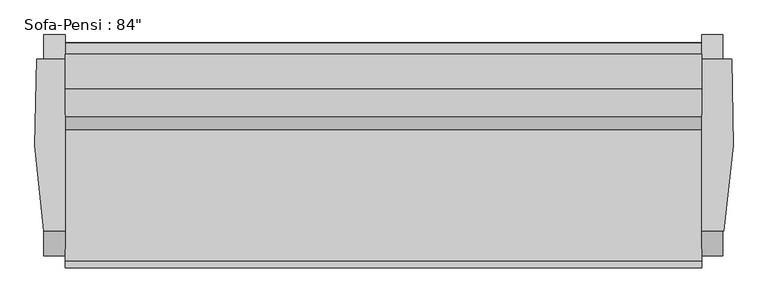
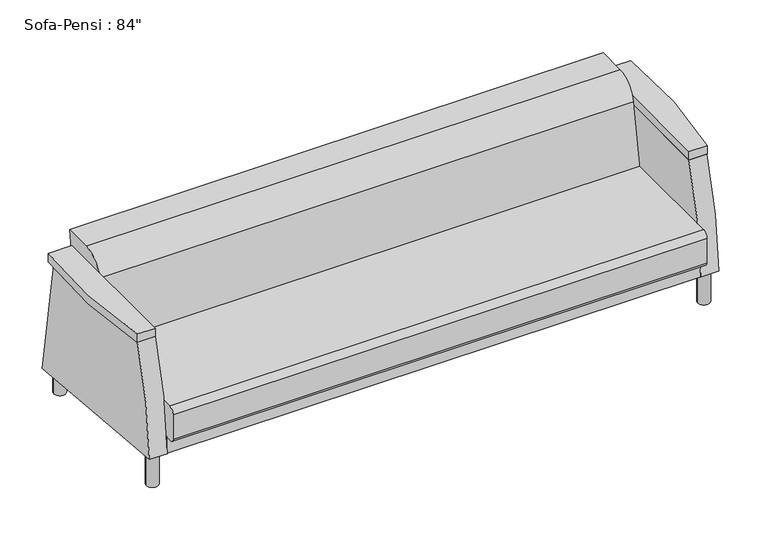
"""IFC4 building model written with IfcOpenShell, lengths in millimetres: furniture geometry."""

from ifc_helpers import new_model, si_unit, point, frame, frame_2d, origin, origin_with_axes, place, context, project, spatial, polyline, circle_curve, trimmed, segment, composite_curve, outline, extrude, source, transform, mapped, element, save


def furniture_1a2ca15e(model_context):
    return source(origin(), model_context, "Body", "SweptSolid", [
        extrude(outline(composite_curve([segment(trimmed(circle_curve(frame_2d((-902.49375, -53.0901639)), 25.4), [point((-927.89375, -53.0901639))], [point((-877.09375, -53.0901639))], False, "CARTESIAN"), True, "CONTINUOUS"), segment(trimmed(circle_curve(frame_2d((-902.49375, -53.0901639)), 25.4), [point((-877.09375, -53.0901639))], [point((-927.89375, -53.0901639))], False, "CARTESIAN"), True, "CONTINUOUS")], self_intersect=False)), origin_with_axes(), (0.0, 0.0, 1.0), 148.43125),
        extrude(outline(composite_curve([segment(trimmed(circle_curve(frame_2d((-902.49375, 632.7098361)), 25.4), [point((-927.89375, 632.7098361))], [point((-877.09375, 632.7098361))], False, "CARTESIAN"), True, "CONTINUOUS"), segment(trimmed(circle_curve(frame_2d((-902.49375, 632.7098361)), 25.4), [point((-877.09375, 632.7098361))], [point((-927.89375, 632.7098361))], False, "CARTESIAN"), True, "CONTINUOUS")], self_intersect=False)), origin_with_axes(), (0.0, 0.0, 1.0), 148.43125),
        extrude(outline(composite_curve([segment(trimmed(circle_curve(frame_2d((1459.70625, 632.7098361)), 25.4), [point((1434.30625, 632.7098361))], [point((1485.10625, 632.7098361))], False, "CARTESIAN"), True, "CONTINUOUS"), segment(trimmed(circle_curve(frame_2d((1459.70625, 632.7098361)), 25.4), [point((1485.10625, 632.7098361))], [point((1434.30625, 632.7098361))], False, "CARTESIAN"), True, "CONTINUOUS")], self_intersect=False)), origin_with_axes(), (0.0, 0.0, 1.0), 148.43125),
        extrude(outline(composite_curve([segment(trimmed(circle_curve(frame_2d((1459.70625, -53.0901639)), 25.4), [point((1434.30625, -53.0901639))], [point((1485.10625, -53.0901639))], False, "CARTESIAN"), True, "CONTINUOUS"), segment(trimmed(circle_curve(frame_2d((1459.70625, -53.0901639)), 25.4), [point((1485.10625, -53.0901639))], [point((1434.30625, -53.0901639))], False, "CARTESIAN"), True, "CONTINUOUS")], self_intersect=False)), origin_with_axes(), (0.0, 0.0, 1.0), 148.43125),
        extrude(outline(polyline([(1421.60625, 668.3047863), (1421.60625, -93.6952137), (-864.39375, -93.6952137), (-864.39375, 668.3047863), (1421.60625, 668.3047863)])), frame((0.0, 0.0, 148.0509954), z_axis=(0.0, 0.0, 1.0), x_axis=(1.0, 0.0, 0.0)), (0.0, 0.0, 1.0), 76.2),
        extrude(outline(composite_curve([segment(polyline([(-9.3943348, 626.0203985), (608.6917937, 626.0203985), (696.2098361, 79.844579), (-97.7900405, 149.3105671)]), True, "CONTINUOUS"), segment(trimmed(circle_curve(frame_2d((1499.9783711, 99.5888442)), 1598.5418814), [point((-97.7900405, 149.3105671))], [point((-9.3943348, 626.0203985))], False, "CARTESIAN"), True, "CONTINUOUS")], self_intersect=False)), frame((-940.59375, 0.0, 0.0), z_axis=(1.0, 0.0, 0.0), x_axis=(0.0, 1.0, 0.0)), (0.0, 0.0, 1.0), 76.2),
        extrude(outline(composite_curve([segment(polyline([(696.2098361, 79.844579), (-97.7900405, 149.3105671)]), True, "CONTINUOUS"), segment(trimmed(circle_curve(frame_2d((1499.9783711, 99.5888442)), 1598.5418814), [point((-97.7900405, 149.3105671))], [point((-9.3943348, 626.0203985))], False, "CARTESIAN"), True, "CONTINUOUS"), segment(polyline([(-9.3943348, 626.0203985), (608.6917937, 626.0203985), (696.2098361, 79.844579)]), True, "CONTINUOUS")], self_intersect=False)), frame((1421.60625, 0.0, 0.0), z_axis=(1.0, 0.0, 0.0), x_axis=(0.0, 1.0, 0.0)), (0.0, 0.0, 1.0), 76.2),
        extrude(outline(composite_curve([segment(trimmed(circle_curve(frame_2d((-116.5901639, 351.2509954)), 25.4), [point((-141.9901639, 351.2509954))], [point((-116.5901639, 376.6509954))], False, "CARTESIAN"), True, "CONTINUOUS"), segment(polyline([(-116.5901639, 376.6509954), (355.3895541, 376.6509954), (402.1988177, 642.1195211)]), True, "CONTINUOUS"), segment(trimmed(circle_curve(frame_2d((502.2552854, 624.4768662)), 101.6), [point((402.1988177, 642.1195211))], [point((502.2552854, 726.0768662))], False, "CARTESIAN"), True, "CONTINUOUS"), segment(polyline([(502.2552854, 726.0768662), (626.3344485, 726.0768662), (609.5377828, 620.1719187), (667.6541767, 224.2509954), (-126.1151639, 224.2509954)]), True, "CONTINUOUS"), segment(trimmed(circle_curve(frame_2d((-126.1151639, 240.1259954)), 15.875), [point((-126.1151639, 224.2509954))], [point((-141.9901639, 240.1259954))], False, "CARTESIAN"), True, "CONTINUOUS"), segment(polyline([(-141.9901639, 240.1259954), (-141.9901639, 351.2509954)]), True, "CONTINUOUS")], self_intersect=False)), frame((-864.39375, 0.0, 0.0), z_axis=(1.0, 0.0, 0.0), x_axis=(0.0, 1.0, 0.0)), (0.0, 0.0, 1.0), 2286.0),
        extrude(outline(composite_curve([segment(polyline([(-864.39375, -9.3943348), (-940.59375, -9.3943348)]), True, "CONTINUOUS"), segment(trimmed(circle_curve(frame_2d((1531.9527561, 401.7789315)), 2506.5014821), [point((-940.59375, -9.3943348))], [point((-965.99375, 608.6917935))], False, "CARTESIAN"), True, "CONTINUOUS"), segment(polyline([(-965.99375, 608.6917935), (-864.39375, 608.6917935), (-864.39375, -9.3943348)]), True, "CONTINUOUS")], self_intersect=False)), frame((0.0, 0.0, 626.0203985), z_axis=(0.0, 0.0, 1.0), x_axis=(1.0, 0.0, 0.0)), (0.0, 0.0, 1.0), 38.1),
        extrude(outline(composite_curve([segment(polyline([(1421.60625, -9.3943348), (1421.60625, 608.9395268), (1530.2864453, 608.9395268)]), True, "CONTINUOUS"), segment(trimmed(circle_curve(frame_2d((-973.7771494, 421.9725391)), 2511.0338789), [point((1530.2864453, 608.9395268))], [point((1499.9273117, -9.3943348))], False, "CARTESIAN"), True, "CONTINUOUS"), segment(polyline([(1499.9273117, -9.3943348), (1421.60625, -9.3943348)]), True, "CONTINUOUS")], self_intersect=False)), frame((0.0, 0.0, 626.0203985), z_axis=(0.0, 0.0, 1.0), x_axis=(1.0, 0.0, 0.0)), (0.0, 0.0, 1.0), 38.1),
    ])


if __name__ == "__main__":
    model = new_model("IFC4")
    model_context = context("Model", 3, world=origin())
    ifc_project = project(units=[si_unit("LENGTHUNIT", "METRE", prefix="MILLI")], contexts=[model_context])
    site = spatial("IfcSite", under=ifc_project)
    building = spatial("IfcBuilding", under=site)
    placement = place(None, origin())
    furniture_shape = furniture_1a2ca15e(model_context)
    element("IfcFurniture", 1, ObjectType="Sofa-Pensi : 84\"", at=placement, inside=building, context=model_context, shape_type="MappedRepresentation", body=[
        mapped(furniture_shape, transform((0.0, 0.0, 0.0), x_axis=(1.0, 0.0, 0.0), y_axis=(0.0, 1.0, 0.0), z_axis=(0.0, 0.0, 1.0))),
    ])
    save(model, "model.ifc")

# Revit data of these elements
# Type "Sofa-Pensi : 84\""
#   Assembly Code = "E2020200"
#   Length = 8' - 0"
#   Frame Material = Cherry
#   Seat Material = Linen, Beige
#   Feet Material = Steel, Chrome Plated
#   Default Elevation = 0
# Element 1 (IfcFurniture, "Sofa-Pensi : 84\"")
#   Materials on its faces: "Cherry", "Linen, Beige", "Steel, Chrome Plated"
# Materials
#   "Cherry": class "Wood", colour RGB 226 177 128, transparency 0, Description = "Prunus Serotina", Cost = 0
#   "Linen, Beige": class "Textile", colour RGB 249 239 230, transparency 0, Description = "Linen, beige", Cost = 0
#   "Steel, Chrome Plated": class "Metal", colour RGB 17 17 17, transparency 0, Description = "Chromiuim plated steel", Cost = 0
